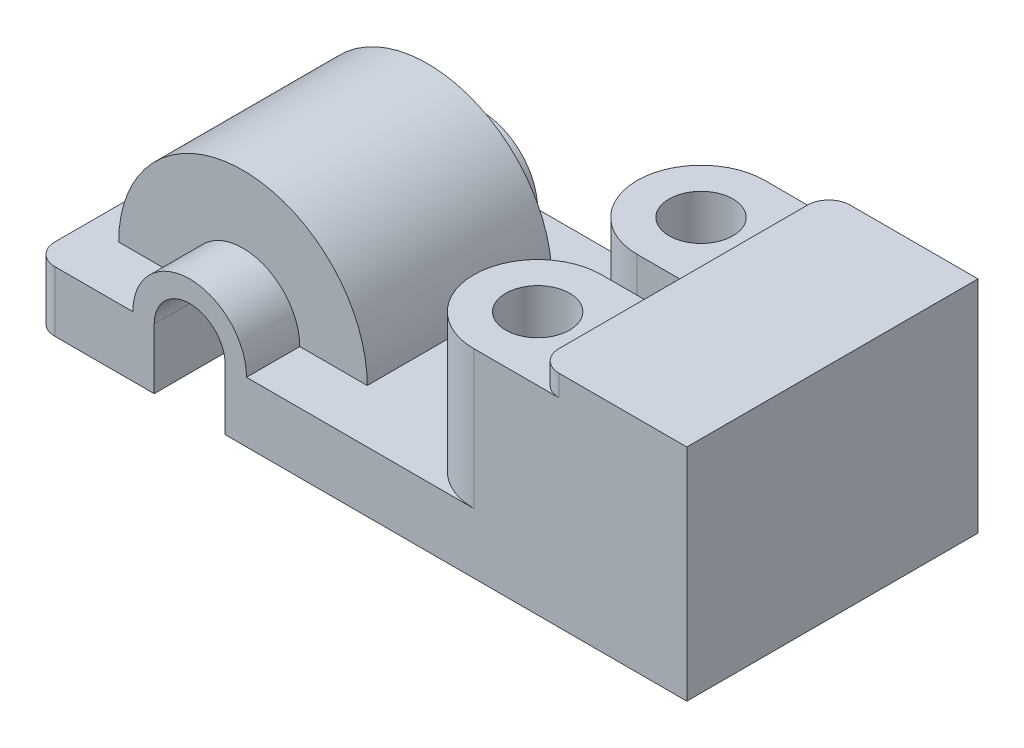
ISO-10303-21;
HEADER;
FILE_DESCRIPTION(('STEP AP214'),'2;1');
FILE_NAME('part.step','',(''),(''),'','','');
FILE_SCHEMA(('AUTOMOTIVE_DESIGN { 1 0 10303 214 1 1 1 1 }'));
ENDSEC;
DATA;
#1=APPLICATION_CONTEXT('core data for automotive mechanical design processes');
#2=APPLICATION_PROTOCOL_DEFINITION('international standard','automotive_design',2000,#1);
#3=PRODUCT_CONTEXT('',#1,'mechanical');
#4=PRODUCT('Part','Part','',(#3));
#5=PRODUCT_RELATED_PRODUCT_CATEGORY('part','',(#4));
#6=PRODUCT_DEFINITION_FORMATION('','',#4);
#7=PRODUCT_DEFINITION_CONTEXT('part definition',#1,'design');
#8=PRODUCT_DEFINITION('design','',#6,#7);
#9=PRODUCT_DEFINITION_SHAPE('','',#8);
#10=(LENGTH_UNIT() NAMED_UNIT(*) SI_UNIT(.MILLI.,.METRE.));
#11=(NAMED_UNIT(*) PLANE_ANGLE_UNIT() SI_UNIT($,.RADIAN.));
#12=(NAMED_UNIT(*) SI_UNIT($,.STERADIAN.) SOLID_ANGLE_UNIT());
#13=UNCERTAINTY_MEASURE_WITH_UNIT(LENGTH_MEASURE(1.E-05),#10,'distance_accuracy_value','');
#14=(GEOMETRIC_REPRESENTATION_CONTEXT(3) GLOBAL_UNCERTAINTY_ASSIGNED_CONTEXT((#13)) GLOBAL_UNIT_ASSIGNED_CONTEXT((#10,
#11,#12)) REPRESENTATION_CONTEXT('',''));
#15=CARTESIAN_POINT('',(0.,0.,0.));
#16=DIRECTION('',(0.,0.,1.));
#17=DIRECTION('',(1.,0.,0.));
#18=AXIS2_PLACEMENT_3D('',#15,#16,#17);
#19=CARTESIAN_POINT('',(-48.,17.,-41.));
#20=DIRECTION('',(0.,0.,1.));
#21=DIRECTION('',(1.,0.,0.));
#22=AXIS2_PLACEMENT_3D('',#19,#20,#21);
#23=CYLINDRICAL_SURFACE('',#22,16.);
#24=DIRECTION('',(0.,0.,1.));
#25=VECTOR('',#24,1.);
#26=CARTESIAN_POINT('',(-64.,17.,-41.));
#27=LINE('',#26,#25);
#28=CARTESIAN_POINT('',(-64.,17.,-41.));
#29=VERTEX_POINT('',#28);
#30=CARTESIAN_POINT('',(-64.,16.9999999999999,-26.));
#31=VERTEX_POINT('',#30);
#32=EDGE_CURVE('E335',#29,#31,#27,.T.);
#33=ORIENTED_EDGE('',*,*,#32,.T.);
#34=CARTESIAN_POINT('',(-48.,17.,-26.));
#35=DIRECTION('',(0.,0.,-1.));
#36=DIRECTION('',(-1.,0.,0.));
#37=AXIS2_PLACEMENT_3D('',#34,#35,#36);
#38=CIRCLE('',#37,16.);
#39=CARTESIAN_POINT('',(-32.,17.,-26.));
#40=VERTEX_POINT('',#39);
#41=EDGE_CURVE('E250',#31,#40,#38,.T.);
#42=ORIENTED_EDGE('',*,*,#41,.T.);
#43=DIRECTION('',(0.,0.,1.));
#44=VECTOR('',#43,1.);
#45=CARTESIAN_POINT('',(-32.,17.,-41.));
#46=LINE('',#45,#44);
#47=CARTESIAN_POINT('',(-32.,17.,-41.));
#48=VERTEX_POINT('',#47);
#49=EDGE_CURVE('E340',#48,#40,#46,.T.);
#50=ORIENTED_EDGE('',*,*,#49,.F.);
#51=CARTESIAN_POINT('',(-48.,17.,-41.));
#52=DIRECTION('',(0.,0.,1.));
#53=DIRECTION('',(1.,0.,0.));
#54=AXIS2_PLACEMENT_3D('',#51,#52,#53);
#55=CIRCLE('',#54,16.);
#56=EDGE_CURVE('E328',#48,#29,#55,.T.);
#57=ORIENTED_EDGE('',*,*,#56,.T.);
#58=EDGE_LOOP('',(#33,#42,#50,#57));
#59=FACE_BOUND('',#58,.T.);
#60=ADVANCED_FACE('F41',(#59),#23,.T.);
#61=CARTESIAN_POINT('',(-86.,0.,-35.));
#62=DIRECTION('',(0.,-1.,0.));
#63=DIRECTION('',(0.,0.,-1.));
#64=AXIS2_PLACEMENT_3D('',#61,#62,#63);
#65=PLANE('',#64);
#66=DIRECTION('',(0.,0.,1.));
#67=VECTOR('',#66,1.);
#68=CARTESIAN_POINT('',(-38.,0.,-41.));
#69=LINE('',#68,#67);
#70=CARTESIAN_POINT('',(-38.,0.,-41.));
#71=VERTEX_POINT('',#70);
#72=CARTESIAN_POINT('',(-38.,0.,41.));
#73=VERTEX_POINT('',#72);
#74=EDGE_CURVE('E325',#71,#73,#69,.T.);
#75=ORIENTED_EDGE('',*,*,#74,.F.);
#76=DIRECTION('',(-1.,0.,0.));
#77=VECTOR('',#76,1.);
#78=CARTESIAN_POINT('',(-86.,0.,-41.));
#79=LINE('',#78,#77);
#80=CARTESIAN_POINT('',(92.,0.,-41.));
#81=VERTEX_POINT('',#80);
#82=EDGE_CURVE('E381',#81,#71,#79,.T.);
#83=ORIENTED_EDGE('',*,*,#82,.F.);
#84=DIRECTION('',(0.,0.,-1.));
#85=VECTOR('',#84,1.);
#86=CARTESIAN_POINT('',(92.,0.,41.));
#87=LINE('',#86,#85);
#88=CARTESIAN_POINT('',(92.,0.,41.));
#89=VERTEX_POINT('',#88);
#90=EDGE_CURVE('E370',#89,#81,#87,.T.);
#91=ORIENTED_EDGE('',*,*,#90,.F.);
#92=DIRECTION('',(1.,0.,0.));
#93=VECTOR('',#92,1.);
#94=CARTESIAN_POINT('',(-86.,0.,41.));
#95=LINE('',#94,#93);
#96=EDGE_CURVE('E393',#73,#89,#95,.T.);
#97=ORIENTED_EDGE('',*,*,#96,.F.);
#98=EDGE_LOOP('',(#75,#83,#91,#97));
#99=FACE_BOUND('',#98,.T.);
#100=ADVANCED_FACE('F481',(#99),#65,.T.);
#101=CARTESIAN_POINT('',(-86.,17.,-35.));
#102=DIRECTION('',(0.,-1.,0.));
#103=DIRECTION('',(0.,0.,-1.));
#104=AXIS2_PLACEMENT_3D('',#101,#102,#103);
#105=PLANE('',#104);
#106=DIRECTION('',(0.,0.,-1.));
#107=VECTOR('',#106,1.);
#108=CARTESIAN_POINT('',(-13.,17.,26.));
#109=LINE('',#108,#107);
#110=CARTESIAN_POINT('',(-13.,17.,26.));
#111=VERTEX_POINT('',#110);
#112=CARTESIAN_POINT('',(-13.,17.,-26.));
#113=VERTEX_POINT('',#112);
#114=EDGE_CURVE('E231',#111,#113,#109,.T.);
#115=ORIENTED_EDGE('',*,*,#114,.F.);
#116=DIRECTION('',(1.,0.,0.));
#117=VECTOR('',#116,1.);
#118=CARTESIAN_POINT('',(-32.,17.,26.));
#119=LINE('',#118,#117);
#120=CARTESIAN_POINT('',(-32.,17.,26.));
#121=VERTEX_POINT('',#120);
#122=EDGE_CURVE('E222',#121,#111,#119,.T.);
#123=ORIENTED_EDGE('',*,*,#122,.F.);
#124=CARTESIAN_POINT('',(-32.,17.,41.));
#125=VERTEX_POINT('',#124);
#126=EDGE_CURVE('E329',#121,#125,#46,.T.);
#127=ORIENTED_EDGE('',*,*,#126,.T.);
#128=DIRECTION('',(1.,0.,0.));
#129=VECTOR('',#128,1.);
#130=CARTESIAN_POINT('',(-86.,17.,41.));
#131=LINE('',#130,#129);
#132=CARTESIAN_POINT('',(32.,17.,41.));
#133=VERTEX_POINT('',#132);
#134=EDGE_CURVE('E380',#125,#133,#131,.T.);
#135=ORIENTED_EDGE('',*,*,#134,.T.);
#136=CARTESIAN_POINT('',(32.,17.,23.));
#137=DIRECTION('',(0.,1.,0.));
#138=DIRECTION('',(0.,0.,1.));
#139=AXIS2_PLACEMENT_3D('',#136,#137,#138);
#140=CIRCLE('',#139,18.);
#141=CARTESIAN_POINT('',(32.,17.,4.99999999999999));
#142=VERTEX_POINT('',#141);
#143=EDGE_CURVE('E251',#142,#133,#140,.T.);
#144=ORIENTED_EDGE('',*,*,#143,.F.);
#145=DIRECTION('',(-1.,0.,0.));
#146=VECTOR('',#145,1.);
#147=CARTESIAN_POINT('',(32.,17.,4.99999999999999));
#148=LINE('',#147,#146);
#149=CARTESIAN_POINT('',(50.,17.,4.99999999999999));
#150=VERTEX_POINT('',#149);
#151=EDGE_CURVE('E261',#150,#142,#148,.T.);
#152=ORIENTED_EDGE('',*,*,#151,.F.);
#153=DIRECTION('',(0.,0.,1.));
#154=VECTOR('',#153,1.);
#155=CARTESIAN_POINT('',(50.,17.,35.));
#156=LINE('',#155,#154);
#157=CARTESIAN_POINT('',(50.,17.,-5.00000000000001));
#158=VERTEX_POINT('',#157);
#159=EDGE_CURVE('E337',#158,#150,#156,.T.);
#160=ORIENTED_EDGE('',*,*,#159,.F.);
#161=DIRECTION('',(1.,0.,0.));
#162=VECTOR('',#161,1.);
#163=CARTESIAN_POINT('',(32.,17.,-5.00000000000001));
#164=LINE('',#163,#162);
#165=CARTESIAN_POINT('',(32.,17.,-5.00000000000001));
#166=VERTEX_POINT('',#165);
#167=EDGE_CURVE('E61',#166,#158,#164,.T.);
#168=ORIENTED_EDGE('',*,*,#167,.F.);
#169=CARTESIAN_POINT('',(32.,17.,-23.));
#170=DIRECTION('',(0.,1.,0.));
#171=DIRECTION('',(0.,0.,1.));
#172=AXIS2_PLACEMENT_3D('',#169,#170,#171);
#173=CIRCLE('',#172,18.);
#174=CARTESIAN_POINT('',(32.,17.,-41.));
#175=VERTEX_POINT('',#174);
#176=EDGE_CURVE('E278',#175,#166,#173,.T.);
#177=ORIENTED_EDGE('',*,*,#176,.F.);
#178=DIRECTION('',(-1.,0.,0.));
#179=VECTOR('',#178,1.);
#180=CARTESIAN_POINT('',(-86.,17.,-41.));
#181=LINE('',#180,#179);
#182=EDGE_CURVE('E368',#175,#48,#181,.T.);
#183=ORIENTED_EDGE('',*,*,#182,.T.);
#184=ORIENTED_EDGE('',*,*,#49,.T.);
#185=DIRECTION('',(1.,0.,0.));
#186=VECTOR('',#185,1.);
#187=CARTESIAN_POINT('',(-32.,17.,-26.));
#188=LINE('',#187,#186);
#189=EDGE_CURVE('E57',#40,#113,#188,.T.);
#190=ORIENTED_EDGE('',*,*,#189,.T.);
#191=EDGE_LOOP('',(#115,#123,#127,#135,#144,#152,#160,#168,#177,#183,#184,#190));
#192=FACE_BOUND('',#191,.T.);
#193=ADVANCED_FACE('F467',(#192),#105,.F.);
#194=CARTESIAN_POINT('',(92.,17.,41.));
#195=DIRECTION('',(-1.,0.,0.));
#196=DIRECTION('',(0.,0.,1.));
#197=AXIS2_PLACEMENT_3D('',#194,#195,#196);
#198=PLANE('',#197);
#199=ORIENTED_EDGE('',*,*,#90,.T.);
#200=DIRECTION('',(0.,-1.,0.));
#201=VECTOR('',#200,1.);
#202=CARTESIAN_POINT('',(92.,17.,-41.));
#203=LINE('',#202,#201);
#204=CARTESIAN_POINT('',(92.,62.,-41.));
#205=VERTEX_POINT('',#204);
#206=EDGE_CURVE('E411',#205,#81,#203,.T.);
#207=ORIENTED_EDGE('',*,*,#206,.F.);
#208=DIRECTION('',(0.,0.,-1.));
#209=VECTOR('',#208,1.);
#210=CARTESIAN_POINT('',(92.,62.,41.));
#211=LINE('',#210,#209);
#212=CARTESIAN_POINT('',(92.,62.,41.));
#213=VERTEX_POINT('',#212);
#214=EDGE_CURVE('E338',#213,#205,#211,.T.);
#215=ORIENTED_EDGE('',*,*,#214,.F.);
#216=DIRECTION('',(0.,-1.,0.));
#217=VECTOR('',#216,1.);
#218=CARTESIAN_POINT('',(92.,17.,41.));
#219=LINE('',#218,#217);
#220=EDGE_CURVE('E379',#213,#89,#219,.T.);
#221=ORIENTED_EDGE('',*,*,#220,.T.);
#222=EDGE_LOOP('',(#199,#207,#215,#221));
#223=FACE_BOUND('',#222,.T.);
#224=ADVANCED_FACE('F43',(#223),#198,.F.);
#225=CARTESIAN_POINT('',(-86.,17.,-41.));
#226=DIRECTION('',(0.,0.,1.));
#227=DIRECTION('',(1.,0.,0.));
#228=AXIS2_PLACEMENT_3D('',#225,#226,#227);
#229=PLANE('',#228);
#230=ORIENTED_EDGE('',*,*,#182,.F.);
#231=DIRECTION('',(0.,-1.,0.));
#232=VECTOR('',#231,1.);
#233=CARTESIAN_POINT('',(32.,56.,-41.));
#234=LINE('',#233,#232);
#235=CARTESIAN_POINT('',(32.,56.,-41.));
#236=VERTEX_POINT('',#235);
#237=EDGE_CURVE('E293',#236,#175,#234,.T.);
#238=ORIENTED_EDGE('',*,*,#237,.F.);
#239=DIRECTION('',(-1.,0.,0.));
#240=VECTOR('',#239,1.);
#241=CARTESIAN_POINT('',(32.,56.,-41.));
#242=LINE('',#241,#240);
#243=CARTESIAN_POINT('',(56.,56.,-41.));
#244=VERTEX_POINT('',#243);
#245=EDGE_CURVE('E286',#244,#236,#242,.T.);
#246=ORIENTED_EDGE('',*,*,#245,.F.);
#247=DIRECTION('',(0.,-1.,0.));
#248=VECTOR('',#247,1.);
#249=CARTESIAN_POINT('',(56.,62.,-41.));
#250=LINE('',#249,#248);
#251=CARTESIAN_POINT('',(56.,62.,-41.));
#252=VERTEX_POINT('',#251);
#253=EDGE_CURVE('E362',#252,#244,#250,.T.);
#254=ORIENTED_EDGE('',*,*,#253,.F.);
#255=DIRECTION('',(-1.,0.,0.));
#256=VECTOR('',#255,1.);
#257=CARTESIAN_POINT('',(92.,62.,-41.));
#258=LINE('',#257,#256);
#259=EDGE_CURVE('E344',#205,#252,#258,.T.);
#260=ORIENTED_EDGE('',*,*,#259,.F.);
#261=ORIENTED_EDGE('',*,*,#206,.T.);
#262=ORIENTED_EDGE('',*,*,#82,.T.);
#263=DIRECTION('',(0.,1.,0.));
#264=VECTOR('',#263,1.);
#265=CARTESIAN_POINT('',(-38.,0.,-41.));
#266=LINE('',#265,#264);
#267=CARTESIAN_POINT('',(-38.,17.,-41.));
#268=VERTEX_POINT('',#267);
#269=EDGE_CURVE('E307',#71,#268,#266,.T.);
#270=ORIENTED_EDGE('',*,*,#269,.T.);
#271=CARTESIAN_POINT('',(-48.,17.,-41.));
#272=DIRECTION('',(0.,0.,1.));
#273=DIRECTION('',(1.,0.,0.));
#274=AXIS2_PLACEMENT_3D('',#271,#272,#273);
#275=CIRCLE('',#274,10.);
#276=CARTESIAN_POINT('',(-58.,17.,-41.));
#277=VERTEX_POINT('',#276);
#278=EDGE_CURVE('E305',#268,#277,#275,.T.);
#279=ORIENTED_EDGE('',*,*,#278,.T.);
#280=DIRECTION('',(0.,-1.,0.));
#281=VECTOR('',#280,1.);
#282=CARTESIAN_POINT('',(-58.,17.,-41.));
#283=LINE('',#282,#281);
#284=CARTESIAN_POINT('',(-58.,0.,-41.));
#285=VERTEX_POINT('',#284);
#286=EDGE_CURVE('E304',#277,#285,#283,.T.);
#287=ORIENTED_EDGE('',*,*,#286,.T.);
#288=CARTESIAN_POINT('',(-86.,0.,-41.));
#289=VERTEX_POINT('',#288);
#290=EDGE_CURVE('E384',#285,#289,#79,.T.);
#291=ORIENTED_EDGE('',*,*,#290,.T.);
#292=DIRECTION('',(0.,-1.,0.));
#293=VECTOR('',#292,1.);
#294=CARTESIAN_POINT('',(-86.,17.,-41.));
#295=LINE('',#294,#293);
#296=CARTESIAN_POINT('',(-86.,17.,-41.));
#297=VERTEX_POINT('',#296);
#298=EDGE_CURVE('E409',#297,#289,#295,.T.);
#299=ORIENTED_EDGE('',*,*,#298,.F.);
#300=EDGE_CURVE('E371',#29,#297,#181,.T.);
#301=ORIENTED_EDGE('',*,*,#300,.F.);
#302=ORIENTED_EDGE('',*,*,#56,.F.);
#303=EDGE_LOOP('',(#230,#238,#246,#254,#260,#261,#262,#270,#279,#287,#291,#299,#301,#302));
#304=FACE_BOUND('',#303,.T.);
#305=ADVANCED_FACE('F438',(#304),#229,.F.);
#306=CARTESIAN_POINT('',(-86.,17.,-35.));
#307=DIRECTION('',(0.,-1.,0.));
#308=DIRECTION('',(0.,0.,-1.));
#309=AXIS2_PLACEMENT_3D('',#306,#307,#308);
#310=CYLINDRICAL_SURFACE('',#309,6.);
#311=CARTESIAN_POINT('',(-86.,0.,-35.));
#312=DIRECTION('',(0.,1.,0.));
#313=DIRECTION('',(0.,0.,-1.));
#314=AXIS2_PLACEMENT_3D('',#311,#312,#313);
#315=CIRCLE('',#314,6.);
#316=CARTESIAN_POINT('',(-92.,0.,-35.));
#317=VERTEX_POINT('',#316);
#318=EDGE_CURVE('E390',#289,#317,#315,.T.);
#319=ORIENTED_EDGE('',*,*,#318,.T.);
#320=DIRECTION('',(0.,-1.,0.));
#321=VECTOR('',#320,1.);
#322=CARTESIAN_POINT('',(-92.,17.,-35.));
#323=LINE('',#322,#321);
#324=CARTESIAN_POINT('',(-92.,17.,-35.));
#325=VERTEX_POINT('',#324);
#326=EDGE_CURVE('E403',#325,#317,#323,.T.);
#327=ORIENTED_EDGE('',*,*,#326,.F.);
#328=CARTESIAN_POINT('',(-86.,17.,-35.));
#329=DIRECTION('',(0.,1.,0.));
#330=DIRECTION('',(0.,0.,-1.));
#331=AXIS2_PLACEMENT_3D('',#328,#329,#330);
#332=CIRCLE('',#331,6.);
#333=EDGE_CURVE('E369',#297,#325,#332,.T.);
#334=ORIENTED_EDGE('',*,*,#333,.F.);
#335=ORIENTED_EDGE('',*,*,#298,.T.);
#336=EDGE_LOOP('',(#319,#327,#334,#335));
#337=FACE_BOUND('',#336,.T.);
#338=ADVANCED_FACE('F502',(#337),#310,.T.);
#339=CARTESIAN_POINT('',(-92.,17.,35.));
#340=DIRECTION('',(1.,0.,0.));
#341=DIRECTION('',(0.,0.,-1.));
#342=AXIS2_PLACEMENT_3D('',#339,#340,#341);
#343=PLANE('',#342);
#344=DIRECTION('',(0.,0.,1.));
#345=VECTOR('',#344,1.);
#346=CARTESIAN_POINT('',(-92.,0.,35.));
#347=LINE('',#346,#345);
#348=CARTESIAN_POINT('',(-92.,0.,35.));
#349=VERTEX_POINT('',#348);
#350=EDGE_CURVE('E386',#317,#349,#347,.T.);
#351=ORIENTED_EDGE('',*,*,#350,.T.);
#352=DIRECTION('',(0.,-1.,0.));
#353=VECTOR('',#352,1.);
#354=CARTESIAN_POINT('',(-92.,17.,35.));
#355=LINE('',#354,#353);
#356=CARTESIAN_POINT('',(-92.,17.,35.));
#357=VERTEX_POINT('',#356);
#358=EDGE_CURVE('E405',#357,#349,#355,.T.);
#359=ORIENTED_EDGE('',*,*,#358,.F.);
#360=DIRECTION('',(0.,0.,1.));
#361=VECTOR('',#360,1.);
#362=CARTESIAN_POINT('',(-92.,17.,35.));
#363=LINE('',#362,#361);
#364=EDGE_CURVE('E373',#325,#357,#363,.T.);
#365=ORIENTED_EDGE('',*,*,#364,.F.);
#366=ORIENTED_EDGE('',*,*,#326,.T.);
#367=EDGE_LOOP('',(#351,#359,#365,#366));
#368=FACE_BOUND('',#367,.T.);
#369=ADVANCED_FACE('F509',(#368),#343,.F.);
#370=CARTESIAN_POINT('',(-86.,17.,35.));
#371=DIRECTION('',(0.,-1.,0.));
#372=DIRECTION('',(0.,0.,-1.));
#373=AXIS2_PLACEMENT_3D('',#370,#371,#372);
#374=CYLINDRICAL_SURFACE('',#373,6.);
#375=CARTESIAN_POINT('',(-86.,0.,35.));
#376=DIRECTION('',(0.,1.,0.));
#377=DIRECTION('',(0.,0.,-1.));
#378=AXIS2_PLACEMENT_3D('',#375,#376,#377);
#379=CIRCLE('',#378,6.);
#380=CARTESIAN_POINT('',(-86.,0.,41.));
#381=VERTEX_POINT('',#380);
#382=EDGE_CURVE('E391',#349,#381,#379,.T.);
#383=ORIENTED_EDGE('',*,*,#382,.T.);
#384=DIRECTION('',(0.,-1.,0.));
#385=VECTOR('',#384,1.);
#386=CARTESIAN_POINT('',(-86.,17.,41.));
#387=LINE('',#386,#385);
#388=CARTESIAN_POINT('',(-86.,17.,41.));
#389=VERTEX_POINT('',#388);
#390=EDGE_CURVE('E396',#389,#381,#387,.T.);
#391=ORIENTED_EDGE('',*,*,#390,.F.);
#392=CARTESIAN_POINT('',(-86.,17.,35.));
#393=DIRECTION('',(0.,1.,0.));
#394=DIRECTION('',(0.,0.,-1.));
#395=AXIS2_PLACEMENT_3D('',#392,#393,#394);
#396=CIRCLE('',#395,6.);
#397=EDGE_CURVE('E374',#357,#389,#396,.T.);
#398=ORIENTED_EDGE('',*,*,#397,.F.);
#399=ORIENTED_EDGE('',*,*,#358,.T.);
#400=EDGE_LOOP('',(#383,#391,#398,#399));
#401=FACE_BOUND('',#400,.T.);
#402=ADVANCED_FACE('F511',(#401),#374,.T.);
#403=CARTESIAN_POINT('',(-86.,17.,41.));
#404=DIRECTION('',(0.,0.,-1.));
#405=DIRECTION('',(-1.,0.,0.));
#406=AXIS2_PLACEMENT_3D('',#403,#404,#405);
#407=PLANE('',#406);
#408=CARTESIAN_POINT('',(-48.,17.,41.));
#409=DIRECTION('',(0.,0.,1.));
#410=DIRECTION('',(1.,0.,0.));
#411=AXIS2_PLACEMENT_3D('',#408,#409,#410);
#412=CIRCLE('',#411,10.);
#413=CARTESIAN_POINT('',(-38.,17.,41.));
#414=VERTEX_POINT('',#413);
#415=CARTESIAN_POINT('',(-58.,17.,41.));
#416=VERTEX_POINT('',#415);
#417=EDGE_CURVE('E301',#414,#416,#412,.T.);
#418=ORIENTED_EDGE('',*,*,#417,.F.);
#419=DIRECTION('',(0.,1.,0.));
#420=VECTOR('',#419,1.);
#421=CARTESIAN_POINT('',(-38.,0.,41.));
#422=LINE('',#421,#420);
#423=EDGE_CURVE('E306',#73,#414,#422,.T.);
#424=ORIENTED_EDGE('',*,*,#423,.F.);
#425=ORIENTED_EDGE('',*,*,#96,.T.);
#426=ORIENTED_EDGE('',*,*,#220,.F.);
#427=DIRECTION('',(1.,0.,0.));
#428=VECTOR('',#427,1.);
#429=CARTESIAN_POINT('',(92.,62.,41.));
#430=LINE('',#429,#428);
#431=CARTESIAN_POINT('',(56.,62.,41.));
#432=VERTEX_POINT('',#431);
#433=EDGE_CURVE('E352',#432,#213,#430,.T.);
#434=ORIENTED_EDGE('',*,*,#433,.F.);
#435=DIRECTION('',(0.,-1.,0.));
#436=VECTOR('',#435,1.);
#437=CARTESIAN_POINT('',(56.,62.,41.));
#438=LINE('',#437,#436);
#439=CARTESIAN_POINT('',(56.,56.,41.));
#440=VERTEX_POINT('',#439);
#441=EDGE_CURVE('E351',#432,#440,#438,.T.);
#442=ORIENTED_EDGE('',*,*,#441,.T.);
#443=DIRECTION('',(1.,0.,0.));
#444=VECTOR('',#443,1.);
#445=CARTESIAN_POINT('',(56.,56.,41.));
#446=LINE('',#445,#444);
#447=CARTESIAN_POINT('',(32.,56.,41.));
#448=VERTEX_POINT('',#447);
#449=EDGE_CURVE('E258',#448,#440,#446,.T.);
#450=ORIENTED_EDGE('',*,*,#449,.F.);
#451=DIRECTION('',(0.,-1.,0.));
#452=VECTOR('',#451,1.);
#453=CARTESIAN_POINT('',(32.,56.,41.));
#454=LINE('',#453,#452);
#455=EDGE_CURVE('E272',#448,#133,#454,.T.);
#456=ORIENTED_EDGE('',*,*,#455,.T.);
#457=ORIENTED_EDGE('',*,*,#134,.F.);
#458=CARTESIAN_POINT('',(-48.,17.,41.));
#459=DIRECTION('',(0.,0.,1.));
#460=DIRECTION('',(1.,0.,0.));
#461=AXIS2_PLACEMENT_3D('',#458,#459,#460);
#462=CIRCLE('',#461,16.);
#463=CARTESIAN_POINT('',(-64.,17.,41.));
#464=VERTEX_POINT('',#463);
#465=EDGE_CURVE('E322',#125,#464,#462,.T.);
#466=ORIENTED_EDGE('',*,*,#465,.T.);
#467=EDGE_CURVE('E377',#389,#464,#131,.T.);
#468=ORIENTED_EDGE('',*,*,#467,.F.);
#469=ORIENTED_EDGE('',*,*,#390,.T.);
#470=CARTESIAN_POINT('',(-58.,0.,41.));
#471=VERTEX_POINT('',#470);
#472=EDGE_CURVE('E392',#381,#471,#95,.T.);
#473=ORIENTED_EDGE('',*,*,#472,.T.);
#474=DIRECTION('',(0.,-1.,0.));
#475=VECTOR('',#474,1.);
#476=CARTESIAN_POINT('',(-58.,17.,41.));
#477=LINE('',#476,#475);
#478=EDGE_CURVE('E314',#416,#471,#477,.T.);
#479=ORIENTED_EDGE('',*,*,#478,.F.);
#480=EDGE_LOOP('',(#418,#424,#425,#426,#434,#442,#450,#456,#457,#466,#468,#469,#473,#479));
#481=FACE_BOUND('',#480,.T.);
#482=ADVANCED_FACE('F426',(#481),#407,.F.);
#483=CARTESIAN_POINT('',(-64.,16.9999999999999,26.));
#484=VERTEX_POINT('',#483);
#485=EDGE_CURVE('E238',#484,#464,#27,.T.);
#486=ORIENTED_EDGE('',*,*,#485,.F.);
#487=DIRECTION('',(1.,0.,0.));
#488=VECTOR('',#487,1.);
#489=CARTESIAN_POINT('',(-83.,17.,26.));
#490=LINE('',#489,#488);
#491=CARTESIAN_POINT('',(-83.,17.,26.));
#492=VERTEX_POINT('',#491);
#493=EDGE_CURVE('E218',#492,#484,#490,.T.);
#494=ORIENTED_EDGE('',*,*,#493,.F.);
#495=DIRECTION('',(0.,0.,-1.));
#496=VECTOR('',#495,1.);
#497=CARTESIAN_POINT('',(-83.,17.,26.));
#498=LINE('',#497,#496);
#499=CARTESIAN_POINT('',(-83.,17.,-26.));
#500=VERTEX_POINT('',#499);
#501=EDGE_CURVE('E227',#492,#500,#498,.T.);
#502=ORIENTED_EDGE('',*,*,#501,.T.);
#503=DIRECTION('',(1.,0.,0.));
#504=VECTOR('',#503,1.);
#505=CARTESIAN_POINT('',(-83.,17.,-26.));
#506=LINE('',#505,#504);
#507=EDGE_CURVE('E244',#500,#31,#506,.T.);
#508=ORIENTED_EDGE('',*,*,#507,.T.);
#509=ORIENTED_EDGE('',*,*,#32,.F.);
#510=ORIENTED_EDGE('',*,*,#300,.T.);
#511=ORIENTED_EDGE('',*,*,#333,.T.);
#512=ORIENTED_EDGE('',*,*,#364,.T.);
#513=ORIENTED_EDGE('',*,*,#397,.T.);
#514=ORIENTED_EDGE('',*,*,#467,.T.);
#515=EDGE_LOOP('',(#486,#494,#502,#508,#509,#510,#511,#512,#513,#514));
#516=FACE_BOUND('',#515,.T.);
#517=ADVANCED_FACE('F236',(#516),#105,.F.);
#518=DIRECTION('',(0.,0.,1.));
#519=VECTOR('',#518,1.);
#520=CARTESIAN_POINT('',(-58.,0.,-41.));
#521=LINE('',#520,#519);
#522=EDGE_CURVE('E321',#285,#471,#521,.T.);
#523=ORIENTED_EDGE('',*,*,#522,.T.);
#524=ORIENTED_EDGE('',*,*,#472,.F.);
#525=ORIENTED_EDGE('',*,*,#382,.F.);
#526=ORIENTED_EDGE('',*,*,#350,.F.);
#527=ORIENTED_EDGE('',*,*,#318,.F.);
#528=ORIENTED_EDGE('',*,*,#290,.F.);
#529=EDGE_LOOP('',(#523,#524,#525,#526,#527,#528));
#530=FACE_BOUND('',#529,.T.);
#531=ADVANCED_FACE('F491',(#530),#65,.T.);
#532=CARTESIAN_POINT('',(56.,62.,-35.));
#533=DIRECTION('',(0.,-1.,0.));
#534=DIRECTION('',(0.,0.,-1.));
#535=AXIS2_PLACEMENT_3D('',#532,#533,#534);
#536=CYLINDRICAL_SURFACE('',#535,6.);
#537=ORIENTED_EDGE('',*,*,#253,.T.);
#538=CARTESIAN_POINT('',(56.,56.,-35.));
#539=DIRECTION('',(0.,1.,0.));
#540=DIRECTION('',(0.,0.,1.));
#541=AXIS2_PLACEMENT_3D('',#538,#539,#540);
#542=CIRCLE('',#541,6.);
#543=CARTESIAN_POINT('',(50.,56.,-35.));
#544=VERTEX_POINT('',#543);
#545=EDGE_CURVE('E299',#244,#544,#542,.T.);
#546=ORIENTED_EDGE('',*,*,#545,.T.);
#547=DIRECTION('',(0.,-1.,0.));
#548=VECTOR('',#547,1.);
#549=CARTESIAN_POINT('',(50.,62.,-35.));
#550=LINE('',#549,#548);
#551=CARTESIAN_POINT('',(50.,62.,-35.));
#552=VERTEX_POINT('',#551);
#553=EDGE_CURVE('E365',#552,#544,#550,.T.);
#554=ORIENTED_EDGE('',*,*,#553,.F.);
#555=CARTESIAN_POINT('',(56.,62.,-35.));
#556=DIRECTION('',(0.,1.,0.));
#557=DIRECTION('',(0.,0.,1.));
#558=AXIS2_PLACEMENT_3D('',#555,#556,#557);
#559=CIRCLE('',#558,6.);
#560=EDGE_CURVE('E343',#252,#552,#559,.T.);
#561=ORIENTED_EDGE('',*,*,#560,.F.);
#562=EDGE_LOOP('',(#537,#546,#554,#561));
#563=FACE_BOUND('',#562,.T.);
#564=ADVANCED_FACE('F443',(#563),#536,.T.);
#565=CARTESIAN_POINT('',(50.,62.,35.));
#566=DIRECTION('',(1.,0.,0.));
#567=DIRECTION('',(0.,0.,-1.));
#568=AXIS2_PLACEMENT_3D('',#565,#566,#567);
#569=PLANE('',#568);
#570=DIRECTION('',(0.,-1.,0.));
#571=VECTOR('',#570,1.);
#572=CARTESIAN_POINT('',(50.,62.,4.99999999999999));
#573=LINE('',#572,#571);
#574=CARTESIAN_POINT('',(50.,56.,4.99999999999999));
#575=VERTEX_POINT('',#574);
#576=EDGE_CURVE('E11',#575,#150,#573,.T.);
#577=ORIENTED_EDGE('',*,*,#576,.F.);
#578=DIRECTION('',(0.,0.,1.));
#579=VECTOR('',#578,1.);
#580=CARTESIAN_POINT('',(50.,56.,35.));
#581=LINE('',#580,#579);
#582=CARTESIAN_POINT('',(50.,56.,35.));
#583=VERTEX_POINT('',#582);
#584=EDGE_CURVE('E271',#575,#583,#581,.T.);
#585=ORIENTED_EDGE('',*,*,#584,.T.);
#586=DIRECTION('',(0.,-1.,0.));
#587=VECTOR('',#586,1.);
#588=CARTESIAN_POINT('',(50.,62.,35.));
#589=LINE('',#588,#587);
#590=CARTESIAN_POINT('',(50.,62.,35.));
#591=VERTEX_POINT('',#590);
#592=EDGE_CURVE('E360',#591,#583,#589,.T.);
#593=ORIENTED_EDGE('',*,*,#592,.F.);
#594=DIRECTION('',(0.,0.,1.));
#595=VECTOR('',#594,1.);
#596=CARTESIAN_POINT('',(50.,62.,35.));
#597=LINE('',#596,#595);
#598=EDGE_CURVE('E350',#552,#591,#597,.T.);
#599=ORIENTED_EDGE('',*,*,#598,.F.);
#600=ORIENTED_EDGE('',*,*,#553,.T.);
#601=DIRECTION('',(0.,0.,1.));
#602=VECTOR('',#601,1.);
#603=CARTESIAN_POINT('',(50.,56.,35.));
#604=LINE('',#603,#602);
#605=CARTESIAN_POINT('',(50.,56.,-5.00000000000001));
#606=VERTEX_POINT('',#605);
#607=EDGE_CURVE('E419',#544,#606,#604,.T.);
#608=ORIENTED_EDGE('',*,*,#607,.T.);
#609=DIRECTION('',(0.,1.,0.));
#610=VECTOR('',#609,1.);
#611=CARTESIAN_POINT('',(50.,62.,-5.00000000000001));
#612=LINE('',#611,#610);
#613=EDGE_CURVE('E412',#158,#606,#612,.T.);
#614=ORIENTED_EDGE('',*,*,#613,.F.);
#615=ORIENTED_EDGE('',*,*,#159,.T.);
#616=EDGE_LOOP('',(#577,#585,#593,#599,#600,#608,#614,#615));
#617=FACE_BOUND('',#616,.T.);
#618=ADVANCED_FACE('F446',(#617),#569,.F.);
#619=CARTESIAN_POINT('',(56.,62.,35.));
#620=DIRECTION('',(0.,-1.,0.));
#621=DIRECTION('',(0.,0.,-1.));
#622=AXIS2_PLACEMENT_3D('',#619,#620,#621);
#623=CYLINDRICAL_SURFACE('',#622,6.);
#624=ORIENTED_EDGE('',*,*,#592,.T.);
#625=CARTESIAN_POINT('',(56.,56.,35.));
#626=DIRECTION('',(0.,1.,0.));
#627=DIRECTION('',(0.,0.,1.));
#628=AXIS2_PLACEMENT_3D('',#625,#626,#627);
#629=CIRCLE('',#628,6.);
#630=EDGE_CURVE('E47',#583,#440,#629,.T.);
#631=ORIENTED_EDGE('',*,*,#630,.T.);
#632=ORIENTED_EDGE('',*,*,#441,.F.);
#633=CARTESIAN_POINT('',(56.,62.,35.));
#634=DIRECTION('',(0.,1.,0.));
#635=DIRECTION('',(0.,0.,-1.));
#636=AXIS2_PLACEMENT_3D('',#633,#634,#635);
#637=CIRCLE('',#636,6.);
#638=EDGE_CURVE('E347',#591,#432,#637,.T.);
#639=ORIENTED_EDGE('',*,*,#638,.F.);
#640=EDGE_LOOP('',(#624,#631,#632,#639));
#641=FACE_BOUND('',#640,.T.);
#642=ADVANCED_FACE('F423',(#641),#623,.T.);
#643=CARTESIAN_POINT('',(56.,62.,-35.));
#644=DIRECTION('',(0.,1.,0.));
#645=DIRECTION('',(0.,0.,1.));
#646=AXIS2_PLACEMENT_3D('',#643,#644,#645);
#647=PLANE('',#646);
#648=ORIENTED_EDGE('',*,*,#214,.T.);
#649=ORIENTED_EDGE('',*,*,#259,.T.);
#650=ORIENTED_EDGE('',*,*,#560,.T.);
#651=ORIENTED_EDGE('',*,*,#598,.T.);
#652=ORIENTED_EDGE('',*,*,#638,.T.);
#653=ORIENTED_EDGE('',*,*,#433,.T.);
#654=EDGE_LOOP('',(#648,#649,#650,#651,#652,#653));
#655=FACE_BOUND('',#654,.T.);
#656=ADVANCED_FACE('F431',(#655),#647,.T.);
#657=CARTESIAN_POINT('',(-48.,17.,26.));
#658=DIRECTION('',(0.,0.,-1.));
#659=DIRECTION('',(-1.,0.,0.));
#660=AXIS2_PLACEMENT_3D('',#657,#658,#659);
#661=CIRCLE('',#660,16.);
#662=EDGE_CURVE('E237',#484,#121,#661,.T.);
#663=ORIENTED_EDGE('',*,*,#662,.F.);
#664=ORIENTED_EDGE('',*,*,#485,.T.);
#665=ORIENTED_EDGE('',*,*,#465,.F.);
#666=ORIENTED_EDGE('',*,*,#126,.F.);
#667=EDGE_LOOP('',(#663,#664,#665,#666));
#668=FACE_BOUND('',#667,.T.);
#669=ADVANCED_FACE('F469',(#668),#23,.T.);
#670=CARTESIAN_POINT('',(-48.,17.,-41.));
#671=DIRECTION('',(0.,0.,1.));
#672=DIRECTION('',(1.,0.,0.));
#673=AXIS2_PLACEMENT_3D('',#670,#671,#672);
#674=CYLINDRICAL_SURFACE('',#673,10.);
#675=ORIENTED_EDGE('',*,*,#417,.T.);
#676=DIRECTION('',(0.,0.,1.));
#677=VECTOR('',#676,1.);
#678=CARTESIAN_POINT('',(-58.,17.,-41.));
#679=LINE('',#678,#677);
#680=EDGE_CURVE('E315',#277,#416,#679,.T.);
#681=ORIENTED_EDGE('',*,*,#680,.F.);
#682=ORIENTED_EDGE('',*,*,#278,.F.);
#683=DIRECTION('',(0.,0.,1.));
#684=VECTOR('',#683,1.);
#685=CARTESIAN_POINT('',(-38.,17.,-41.));
#686=LINE('',#685,#684);
#687=EDGE_CURVE('E316',#268,#414,#686,.T.);
#688=ORIENTED_EDGE('',*,*,#687,.T.);
#689=EDGE_LOOP('',(#675,#681,#682,#688));
#690=FACE_BOUND('',#689,.T.);
#691=ADVANCED_FACE('F472',(#690),#674,.F.);
#692=CARTESIAN_POINT('',(-38.,0.,-41.));
#693=DIRECTION('',(1.,0.,0.));
#694=DIRECTION('',(0.,0.,-1.));
#695=AXIS2_PLACEMENT_3D('',#692,#693,#694);
#696=PLANE('',#695);
#697=ORIENTED_EDGE('',*,*,#423,.T.);
#698=ORIENTED_EDGE('',*,*,#687,.F.);
#699=ORIENTED_EDGE('',*,*,#269,.F.);
#700=ORIENTED_EDGE('',*,*,#74,.T.);
#701=EDGE_LOOP('',(#697,#698,#699,#700));
#702=FACE_BOUND('',#701,.T.);
#703=ADVANCED_FACE('F478',(#702),#696,.F.);
#704=CARTESIAN_POINT('',(-58.,17.,-41.));
#705=DIRECTION('',(-1.,0.,0.));
#706=DIRECTION('',(0.,0.,1.));
#707=AXIS2_PLACEMENT_3D('',#704,#705,#706);
#708=PLANE('',#707);
#709=ORIENTED_EDGE('',*,*,#478,.T.);
#710=ORIENTED_EDGE('',*,*,#522,.F.);
#711=ORIENTED_EDGE('',*,*,#286,.F.);
#712=ORIENTED_EDGE('',*,*,#680,.T.);
#713=EDGE_LOOP('',(#709,#710,#711,#712));
#714=FACE_BOUND('',#713,.T.);
#715=ADVANCED_FACE('F518',(#714),#708,.F.);
#716=CARTESIAN_POINT('',(32.,56.,-23.));
#717=DIRECTION('',(0.,1.,0.));
#718=DIRECTION('',(0.,0.,1.));
#719=AXIS2_PLACEMENT_3D('',#716,#717,#718);
#720=PLANE('',#719);
#721=CARTESIAN_POINT('',(32.,56.,-23.));
#722=DIRECTION('',(0.,1.,0.));
#723=DIRECTION('',(0.,0.,1.));
#724=AXIS2_PLACEMENT_3D('',#721,#722,#723);
#725=CIRCLE('',#724,9.);
#726=CARTESIAN_POINT('',(32.,56.,-14.));
#727=VERTEX_POINT('',#726);
#728=EDGE_CURVE('E280',#727,#727,#725,.T.);
#729=ORIENTED_EDGE('',*,*,#728,.F.);
#730=EDGE_LOOP('',(#729));
#731=FACE_BOUND('',#730,.T.);
#732=ORIENTED_EDGE('',*,*,#545,.F.);
#733=ORIENTED_EDGE('',*,*,#245,.T.);
#734=CARTESIAN_POINT('',(32.,56.,-23.));
#735=DIRECTION('',(0.,1.,0.));
#736=DIRECTION('',(0.,0.,1.));
#737=AXIS2_PLACEMENT_3D('',#734,#735,#736);
#738=CIRCLE('',#737,18.);
#739=CARTESIAN_POINT('',(32.,56.,-5.00000000000001));
#740=VERTEX_POINT('',#739);
#741=EDGE_CURVE('E283',#236,#740,#738,.T.);
#742=ORIENTED_EDGE('',*,*,#741,.T.);
#743=DIRECTION('',(1.,0.,0.));
#744=VECTOR('',#743,1.);
#745=CARTESIAN_POINT('',(32.,56.,-5.00000000000001));
#746=LINE('',#745,#744);
#747=EDGE_CURVE('E287',#740,#606,#746,.T.);
#748=ORIENTED_EDGE('',*,*,#747,.T.);
#749=ORIENTED_EDGE('',*,*,#607,.F.);
#750=EDGE_LOOP('',(#732,#733,#742,#748,#749));
#751=FACE_BOUND('',#750,.T.);
#752=ADVANCED_FACE('F532',(#731,#751),#720,.T.);
#753=CARTESIAN_POINT('',(32.,56.,-5.00000000000001));
#754=DIRECTION('',(0.,0.,-1.));
#755=DIRECTION('',(-1.,0.,0.));
#756=AXIS2_PLACEMENT_3D('',#753,#754,#755);
#757=PLANE('',#756);
#758=ORIENTED_EDGE('',*,*,#167,.T.);
#759=ORIENTED_EDGE('',*,*,#613,.T.);
#760=ORIENTED_EDGE('',*,*,#747,.F.);
#761=DIRECTION('',(0.,-1.,0.));
#762=VECTOR('',#761,1.);
#763=CARTESIAN_POINT('',(32.,56.,-5.00000000000001));
#764=LINE('',#763,#762);
#765=EDGE_CURVE('E300',#740,#166,#764,.T.);
#766=ORIENTED_EDGE('',*,*,#765,.T.);
#767=EDGE_LOOP('',(#758,#759,#760,#766));
#768=FACE_BOUND('',#767,.T.);
#769=ADVANCED_FACE('F539',(#768),#757,.F.);
#770=CARTESIAN_POINT('',(32.,56.,-23.));
#771=DIRECTION('',(0.,-1.,0.));
#772=DIRECTION('',(0.,0.,-1.));
#773=AXIS2_PLACEMENT_3D('',#770,#771,#772);
#774=CYLINDRICAL_SURFACE('',#773,18.);
#775=ORIENTED_EDGE('',*,*,#176,.T.);
#776=ORIENTED_EDGE('',*,*,#765,.F.);
#777=ORIENTED_EDGE('',*,*,#741,.F.);
#778=ORIENTED_EDGE('',*,*,#237,.T.);
#779=EDGE_LOOP('',(#775,#776,#777,#778));
#780=FACE_BOUND('',#779,.T.);
#781=ADVANCED_FACE('F534',(#780),#774,.T.);
#782=CARTESIAN_POINT('',(32.,56.,-23.));
#783=DIRECTION('',(0.,-1.,0.));
#784=DIRECTION('',(0.,0.,-1.));
#785=AXIS2_PLACEMENT_3D('',#782,#783,#784);
#786=CYLINDRICAL_SURFACE('',#785,9.);
#787=ORIENTED_EDGE('',*,*,#728,.T.);
#788=EDGE_LOOP('',(#787));
#789=FACE_BOUND('',#788,.T.);
#790=CARTESIAN_POINT('',(32.,17.,-23.));
#791=DIRECTION('',(0.,1.,0.));
#792=DIRECTION('',(0.,0.,1.));
#793=AXIS2_PLACEMENT_3D('',#790,#791,#792);
#794=CIRCLE('',#793,9.);
#795=CARTESIAN_POINT('',(32.,17.,-14.));
#796=VERTEX_POINT('',#795);
#797=EDGE_CURVE('E277',#796,#796,#794,.T.);
#798=ORIENTED_EDGE('',*,*,#797,.F.);
#799=EDGE_LOOP('',(#798));
#800=FACE_BOUND('',#799,.T.);
#801=ADVANCED_FACE('F540',(#789,#800),#786,.F.);
#802=ORIENTED_EDGE('',*,*,#797,.T.);
#803=EDGE_LOOP('',(#802));
#804=FACE_BOUND('',#803,.T.);
#805=ADVANCED_FACE('F550',(#804),#105,.F.);
#806=CARTESIAN_POINT('',(32.,56.,4.99999999999999));
#807=DIRECTION('',(0.,0.,1.));
#808=DIRECTION('',(1.,0.,0.));
#809=AXIS2_PLACEMENT_3D('',#806,#807,#808);
#810=PLANE('',#809);
#811=DIRECTION('',(-1.,0.,0.));
#812=VECTOR('',#811,1.);
#813=CARTESIAN_POINT('',(32.,56.,4.99999999999999));
#814=LINE('',#813,#812);
#815=CARTESIAN_POINT('',(32.,56.,4.99999999999999));
#816=VERTEX_POINT('',#815);
#817=EDGE_CURVE('E263',#575,#816,#814,.T.);
#818=ORIENTED_EDGE('',*,*,#817,.F.);
#819=ORIENTED_EDGE('',*,*,#576,.T.);
#820=ORIENTED_EDGE('',*,*,#151,.T.);
#821=DIRECTION('',(0.,-1.,0.));
#822=VECTOR('',#821,1.);
#823=CARTESIAN_POINT('',(32.,56.,4.99999999999999));
#824=LINE('',#823,#822);
#825=EDGE_CURVE('E264',#816,#142,#824,.T.);
#826=ORIENTED_EDGE('',*,*,#825,.F.);
#827=EDGE_LOOP('',(#818,#819,#820,#826));
#828=FACE_BOUND('',#827,.T.);
#829=ADVANCED_FACE('F453',(#828),#810,.F.);
#830=CARTESIAN_POINT('',(32.,56.,23.));
#831=DIRECTION('',(0.,1.,0.));
#832=DIRECTION('',(0.,0.,1.));
#833=AXIS2_PLACEMENT_3D('',#830,#831,#832);
#834=PLANE('',#833);
#835=ORIENTED_EDGE('',*,*,#584,.F.);
#836=ORIENTED_EDGE('',*,*,#817,.T.);
#837=CARTESIAN_POINT('',(32.,56.,23.));
#838=DIRECTION('',(0.,1.,0.));
#839=DIRECTION('',(0.,0.,1.));
#840=AXIS2_PLACEMENT_3D('',#837,#838,#839);
#841=CIRCLE('',#840,18.);
#842=EDGE_CURVE('E260',#816,#448,#841,.T.);
#843=ORIENTED_EDGE('',*,*,#842,.T.);
#844=ORIENTED_EDGE('',*,*,#449,.T.);
#845=ORIENTED_EDGE('',*,*,#630,.F.);
#846=EDGE_LOOP('',(#835,#836,#843,#844,#845));
#847=FACE_BOUND('',#846,.T.);
#848=CARTESIAN_POINT('',(32.,56.,23.));
#849=DIRECTION('',(0.,1.,0.));
#850=DIRECTION('',(0.,0.,1.));
#851=AXIS2_PLACEMENT_3D('',#848,#849,#850);
#852=CIRCLE('',#851,9.);
#853=CARTESIAN_POINT('',(32.,56.,32.));
#854=VERTEX_POINT('',#853);
#855=EDGE_CURVE('E252',#854,#854,#852,.T.);
#856=ORIENTED_EDGE('',*,*,#855,.F.);
#857=EDGE_LOOP('',(#856));
#858=FACE_BOUND('',#857,.T.);
#859=ADVANCED_FACE('F452',(#847,#858),#834,.T.);
#860=CARTESIAN_POINT('',(32.,56.,23.));
#861=DIRECTION('',(0.,-1.,0.));
#862=DIRECTION('',(0.,0.,-1.));
#863=AXIS2_PLACEMENT_3D('',#860,#861,#862);
#864=CYLINDRICAL_SURFACE('',#863,18.);
#865=ORIENTED_EDGE('',*,*,#143,.T.);
#866=ORIENTED_EDGE('',*,*,#455,.F.);
#867=ORIENTED_EDGE('',*,*,#842,.F.);
#868=ORIENTED_EDGE('',*,*,#825,.T.);
#869=EDGE_LOOP('',(#865,#866,#867,#868));
#870=FACE_BOUND('',#869,.T.);
#871=ADVANCED_FACE('F462',(#870),#864,.T.);
#872=CARTESIAN_POINT('',(32.,56.,23.));
#873=DIRECTION('',(0.,-1.,0.));
#874=DIRECTION('',(0.,0.,-1.));
#875=AXIS2_PLACEMENT_3D('',#872,#873,#874);
#876=CYLINDRICAL_SURFACE('',#875,9.);
#877=ORIENTED_EDGE('',*,*,#855,.T.);
#878=EDGE_LOOP('',(#877));
#879=FACE_BOUND('',#878,.T.);
#880=CARTESIAN_POINT('',(32.,17.,23.));
#881=DIRECTION('',(0.,1.,0.));
#882=DIRECTION('',(0.,0.,1.));
#883=AXIS2_PLACEMENT_3D('',#880,#881,#882);
#884=CIRCLE('',#883,9.);
#885=CARTESIAN_POINT('',(32.,17.,32.));
#886=VERTEX_POINT('',#885);
#887=EDGE_CURVE('E235',#886,#886,#884,.T.);
#888=ORIENTED_EDGE('',*,*,#887,.F.);
#889=EDGE_LOOP('',(#888));
#890=FACE_BOUND('',#889,.T.);
#891=ADVANCED_FACE('F552',(#879,#890),#876,.F.);
#892=ORIENTED_EDGE('',*,*,#887,.T.);
#893=EDGE_LOOP('',(#892));
#894=FACE_BOUND('',#893,.T.);
#895=ADVANCED_FACE('F559',(#894),#105,.F.);
#896=CARTESIAN_POINT('',(-48.,17.,26.));
#897=DIRECTION('',(0.,0.,-1.));
#898=DIRECTION('',(-1.,0.,0.));
#899=AXIS2_PLACEMENT_3D('',#896,#897,#898);
#900=CYLINDRICAL_SURFACE('',#899,35.);
#901=CARTESIAN_POINT('',(-48.,17.,-26.));
#902=DIRECTION('',(0.,0.,1.));
#903=DIRECTION('',(1.,0.,0.));
#904=AXIS2_PLACEMENT_3D('',#901,#902,#903);
#905=CIRCLE('',#904,35.);
#906=EDGE_CURVE('E230',#113,#500,#905,.T.);
#907=ORIENTED_EDGE('',*,*,#906,.T.);
#908=ORIENTED_EDGE('',*,*,#501,.F.);
#909=CARTESIAN_POINT('',(-48.,17.,26.));
#910=DIRECTION('',(0.,0.,1.));
#911=DIRECTION('',(1.,0.,0.));
#912=AXIS2_PLACEMENT_3D('',#909,#910,#911);
#913=CIRCLE('',#912,35.);
#914=EDGE_CURVE('E211',#111,#492,#913,.T.);
#915=ORIENTED_EDGE('',*,*,#914,.F.);
#916=ORIENTED_EDGE('',*,*,#114,.T.);
#917=EDGE_LOOP('',(#907,#908,#915,#916));
#918=FACE_BOUND('',#917,.T.);
#919=ADVANCED_FACE('F226',(#918),#900,.T.);
#920=CARTESIAN_POINT('',(-48.,17.,26.));
#921=DIRECTION('',(0.,0.,1.));
#922=DIRECTION('',(1.,0.,0.));
#923=AXIS2_PLACEMENT_3D('',#920,#921,#922);
#924=PLANE('',#923);
#925=ORIENTED_EDGE('',*,*,#914,.T.);
#926=ORIENTED_EDGE('',*,*,#493,.T.);
#927=ORIENTED_EDGE('',*,*,#662,.T.);
#928=ORIENTED_EDGE('',*,*,#122,.T.);
#929=EDGE_LOOP('',(#925,#926,#927,#928));
#930=FACE_BOUND('',#929,.T.);
#931=ADVANCED_FACE('F216',(#930),#924,.T.);
#932=CARTESIAN_POINT('',(-48.,17.,-26.));
#933=DIRECTION('',(0.,0.,1.));
#934=DIRECTION('',(1.,0.,0.));
#935=AXIS2_PLACEMENT_3D('',#932,#933,#934);
#936=PLANE('',#935);
#937=ORIENTED_EDGE('',*,*,#906,.F.);
#938=ORIENTED_EDGE('',*,*,#189,.F.);
#939=ORIENTED_EDGE('',*,*,#41,.F.);
#940=ORIENTED_EDGE('',*,*,#507,.F.);
#941=EDGE_LOOP('',(#937,#938,#939,#940));
#942=FACE_BOUND('',#941,.T.);
#943=ADVANCED_FACE('F565',(#942),#936,.F.);
#944=CLOSED_SHELL('',(#60,#100,#193,#224,#305,#338,#369,#402,#482,#517,#531,#564,#618,#642,#656,
#669,#691,#703,#715,#752,#769,#781,#801,#805,#829,#859,#871,#891,#895,#919,#931,#943));
#945=MANIFOLD_SOLID_BREP('B2',#944);
#946=ADVANCED_BREP_SHAPE_REPRESENTATION('',(#18,#945),#14);
#947=SHAPE_DEFINITION_REPRESENTATION(#9,#946);
ENDSEC;
END-ISO-10303-21;
